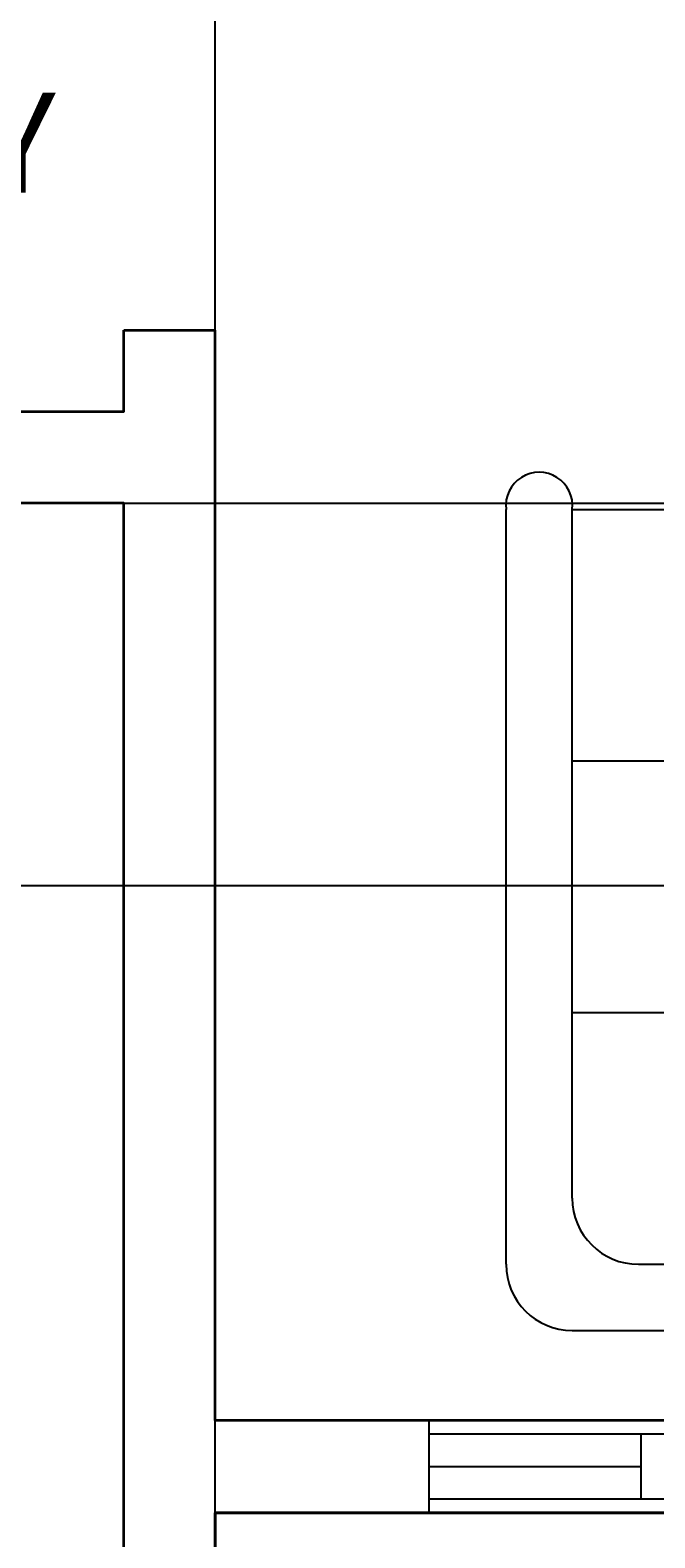
# Model space of a CAD drawing. Units: millimetres. Extents: x 19292 to 100733, y 12374 to 26974.
# Tile 3 of 24: x 26744 to 28279, y 14845 to 18550. Entities that reach past the tile are written whole.
import ezdxf

# ---------------------------------------------------------------- set-up
doc = ezdxf.new("R2010")
doc.units = ezdxf.units.MM
for name, color, linetype, lineweight in [('A-ANNO-DIMS', 2, 'Continuous', 18), ('A-AREA-IDEN', 3, 'Continuous', 25), ('A-FLOR-PATT', 252, 'Continuous', 13), ('A-FURN', 8, 'Continuous', 18), ('A-GLAZ', 3, 'Continuous', 25), ('A-WALL', 7, 'Continuous', 35)]:
    doc.layers.add(name, color=color, linetype=linetype, lineweight=lineweight)
doc.layers.add('FURNITURE', color=40, linetype='Continuous')
doc.layers.add('WINDOWS', color=50, linetype='Continuous')
doc.styles.get("Standard").update_dxf_attribs({"font": 'arial.ttf'})
doc.dimstyles.get("Standard").update_dxf_attribs({"dimtxt": 0.18, "dimasz": 0.18, "dimexe": 0.18, "dimexo": 0.0625, "dimgap": 0.09, "dimtad": 0, "dimtih": 1, "dimtoh": 1, "dimdec": 4, "dimzin": 0, "dimdsep": 46, "dimtxsty": 'Standard', "dimcen": 0.09, "dimadec": 0, "dimazin": 0, "dimtfac": 1, "dimtdec": 4, "dimtofl": 0, "dimtmove": 0, "dimatfit": 3, "dimfxl": 1, "dimtolj": 1, "dimtzin": 0, "dimarcsym": 0})

# ---------------------------------------------------------------- blocks, each defined once
blk = doc.blocks.new('WW')
at = {"layer": 'WINDOWS'}
for p, q in [((-5183.9, -4940.9), (-3983.9, -4940.9)), ((-4663.9, -4940.9), (-4663.9, -5100.9)), ((-4503.9, -4940.9), (-4503.9, -5100.9)), ((-4503.9, -4940.9), (-4503.9, -5100.9)), ((-5183.9, -5020.9), (-4663.9, -5020.9)), ((-4503.9, -5020.9), (-3983.9, -5020.9)), ((-5183.9, -5100.9), (-3983.9, -5100.9))]:
    blk.add_line(p, q, dxfattribs=at)
for points in [[(-5183.9, -5133.4), (-5183.9, -4908.4)], [(-3983.9, -4908.4), (-3983.9, -5133.4)]]:
    blk.add_lwpolyline(points, dxfattribs=at)
blk = doc.blocks.new('2sofa-hf')
at = {"layer": 'FURNITURE'}
for p, q in [((-27, -29.85), (-27, 31.72)), ((-21.6, -24.45), (-21.6, 31.72)), ((-21.6, 31.72), (-13.69, 31.72)), ((0, -6.32), (0, 19.35)), ((-21.62, 11.2), (-0.02, 11.2)), ((-21.57, -9.32), (-2.97, -9.32)), ((0, -23.85), (0, -12.32)), ((-16.2, -29.85), (-3, -29.85)), ((-21.6, -35.25), (-2.43, -35.25))]:
    blk.add_line(p, q, dxfattribs=at)
for centre, radius, start, end in [((-24.3, 32.03), 2.72, 353.479, 186.521), ((-11.92, 19.92), 11.93, 357.2261, 98.5207), ((-3, -6.32), 3, 270, 0), ((-3, -12.32), 3, 0, 90), ((-16.2, -24.45), 5.4, 180, 270), ((-6, -23.85), 6, 270, 0), ((-21.6, -29.85), 5.4, 180, 270), ((-2.71, -32.55), 2.72, 263.9744, 96.0256)]:
    blk.add_arc(centre, radius, start, end, dxfattribs=at)
blk = doc.blocks.new('*D70')
at = {"layer": 'A-ANNO-DIMS', "color": 0, "lineweight": -2, "transparency": 16777216}
for p, q in [((23573.9, 17387.7), (36879.3, 17387.7)), ((36879.2, 17387.6), (36879.2, 16917.9)), ((36879.2, 16447.9), (36879.2, 16917.6)), ((23573.9, 16447.7), (36879.3, 16447.7))]:
    blk.add_line(p, q, dxfattribs=at)
at = {"layer": 'A-ANNO-DIMS', "color": 0, "transparency": 16777216}
for points in [[(36879.1, 17387.6), (36879.2, 17387.6), (36879.2, 17387.7)], [(36879.1, 16447.9), (36879.2, 16447.9), (36879.2, 16447.7)]]:
    blk.add_solid(points, dxfattribs=at)
at = {"layer": 'Defpoints', "color": 0, "transparency": 16777216}
for p in [(23573.8, 17387.7), (36879.2, 17387.7), (23573.8, 16447.7)]:
    blk.add_point(p, dxfattribs=at)
at = {"layer": 'A-ANNO-DIMS', "color": 0, "transparency": 16777216, "insert": (36879.2, 16917.7), "char_height": 0.18, "attachment_point": 5}
blk.add_mtext('\\A1;940', dxfattribs=at)
blk = doc.blocks.new('*D71')
at = {"layer": 'A-ANNO-DIMS', "color": 0, "lineweight": -2, "transparency": 16777216}
for p, q in [((26973.8, 17387.7), (26278.6, 17387.7)), ((26278.8, 17387.6), (26278.8, 15587.9)), ((26278.8, 13787.9), (26278.8, 15587.6)), ((26973.8, 13787.7), (26278.6, 13787.7))]:
    blk.add_line(p, q, dxfattribs=at)
at = {"layer": 'A-ANNO-DIMS', "color": 0, "transparency": 16777216}
for points in [[(26278.8, 17387.6), (26278.8, 17387.6), (26278.8, 17387.7)], [(26278.8, 13787.9), (26278.8, 13787.9), (26278.8, 13787.7)]]:
    blk.add_solid(points, dxfattribs=at)
at = {"layer": 'Defpoints', "color": 0, "transparency": 16777216}
for p in [(26278.8, 17387.7), (26973.8, 17387.7), (26973.8, 13787.7)]:
    blk.add_point(p, dxfattribs=at)
at = {"layer": 'A-ANNO-DIMS', "color": 0, "transparency": 16777216, "insert": (26278.8, 15587.7), "char_height": 0.18, "attachment_point": 5}
blk.add_mtext('\\A1;3600', dxfattribs=at)
blk = doc.blocks.new('*D79')
at = {"layer": 'A-ANNO-DIMS', "color": 0, "lineweight": -2, "transparency": 16777216}
for p, q in [((22694.1, 22860.7), (22694.1, 12808.8)), ((36144.2, 15985.7), (36144.2, 12808.8)), ((22694.3, 12809), (29418.7, 12809)), ((36144, 12809), (29419.6, 12809))]:
    blk.add_line(p, q, dxfattribs=at)
at = {"layer": 'A-ANNO-DIMS', "color": 0, "transparency": 16777216}
for points in [[(22694.3, 12809), (22694.3, 12809), (22694.1, 12809)], [(36144, 12809), (36144, 12809), (36144.2, 12809)]]:
    blk.add_solid(points, dxfattribs=at)
at = {"layer": 'Defpoints', "color": 0, "transparency": 16777216}
for p in [(22694.1, 22860.7), (36144.2, 15985.7), (36144.2, 12809)]:
    blk.add_point(p, dxfattribs=at)
at = {"layer": 'A-ANNO-DIMS', "color": 0, "transparency": 16777216, "insert": (29419.2, 12809), "char_height": 0.18, "attachment_point": 5}
blk.add_mtext('\\A1;13450', dxfattribs=at)
blk = doc.blocks.new('*D82')
at = {"layer": 'A-ANNO-DIMS', "color": 0, "lineweight": -2, "transparency": 16777216}
for p, q in [((27198.8, 13562.8), (27198.8, 23555.9)), ((27199, 23555.7), (29296.4, 23555.7)), ((31394.6, 23555.7), (29297.2, 23555.7)), ((31394.8, 13544.1), (31394.8, 23555.9))]:
    blk.add_line(p, q, dxfattribs=at)
at = {"layer": 'A-ANNO-DIMS', "color": 0, "transparency": 16777216}
for points in [[(27199, 23555.8), (27199, 23555.7), (27198.8, 23555.7)], [(31394.6, 23555.8), (31394.6, 23555.7), (31394.8, 23555.7)]]:
    blk.add_solid(points, dxfattribs=at)
at = {"layer": 'Defpoints', "color": 0, "transparency": 16777216}
for p in [(31394.8, 23555.7), (27198.8, 13562.7), (31394.8, 13544)]:
    blk.add_point(p, dxfattribs=at)
at = {"layer": 'A-ANNO-DIMS', "color": 0, "transparency": 16777216, "insert": (29296.8, 23555.7), "char_height": 0.18, "attachment_point": 5}
blk.add_mtext('\\A1;4196', dxfattribs=at)
blk = doc.blocks.new('*D86')
at = {"layer": 'A-ANNO-DIMS', "color": 0, "lineweight": -2, "transparency": 16777216}
for p, q in [((27198.8, 15132.8), (27198.8, 23555.9)), ((27199, 23555.7), (29198.5, 23555.7)), ((31198.6, 23555.7), (29199.2, 23555.7)), ((31198.8, 15132.8), (31198.8, 23555.9))]:
    blk.add_line(p, q, dxfattribs=at)
at = {"layer": 'A-ANNO-DIMS', "color": 0, "transparency": 16777216}
for points in [[(27199, 23555.8), (27199, 23555.7), (27198.8, 23555.7)], [(31198.6, 23555.8), (31198.6, 23555.7), (31198.8, 23555.7)]]:
    blk.add_solid(points, dxfattribs=at)
at = {"layer": 'Defpoints', "color": 0, "transparency": 16777216}
for p in [(31198.8, 23555.7), (27198.8, 15132.7), (31198.8, 15132.7)]:
    blk.add_point(p, dxfattribs=at)
at = {"layer": 'A-ANNO-DIMS', "color": 0, "transparency": 16777216, "insert": (29198.8, 23555.7), "char_height": 0.18, "attachment_point": 5}
blk.add_mtext('\\A1;4000', dxfattribs=at)

msp = doc.modelspace()

# ---------------------------------------------------------------- hatches: boundary and pattern name
at = {"layer": 'A-FLOR-PATT'}
h = msp.add_hatch(dxfattribs=at)
h.set_pattern_fill('CROSS', color=256, scale=40)
h.paths.add_polyline_path([(31394.799, 14906.403), (31051.542, 14906.403), (29468.571, 14906.403), (27198.815, 14906.403), (27198.815, 13543.993), (31394.799, 13543.993)])
h.paths.add_polyline_path([(27828.096, 14036.581), (30629.164, 14036.581), (30629.164, 14443.478), (27828.096, 14443.478)], flags=24)

# ---------------------------------------------------------------- linework, layer by layer
at = {"layer": 'A-WALL'}
msp.add_line((26973.815, 17812.748), (27198.815, 17812.748), dxfattribs=at)
for points in [[(29548.571, 14906.403), (27198.815, 14906.403), (27198.815, 13562.748), (23348.815, 13562.748), (23348.815, 19010.725), (22694.132, 19010.725), (22694.132, 22860.725), (28369.132, 22860.725), (28369.132, 21460.725), (31169.132, 21460.725), (31169.132, 22460.725), (34419.132, 22460.725), (34419.132, 22208.026)], [(26576.145, 17612.748), (26973.815, 17612.748), (26973.815, 17812.748)], [(29468.571, 15132.748), (27198.815, 15132.748), (27198.815, 17812.748)], [(25756.145, 17387.748), (23573.815, 17387.748), (23573.815, 13787.748), (26973.815, 13787.748), (26973.815, 17387.748), (26656.145, 17387.748)], [(31051.542, 14906.403), (31394.799, 14906.403), (31394.799, 13543.993), (27198.815, 13543.993), (27198.815, 14906.403), (29548.571, 14906.403)]]:
    msp.add_lwpolyline(points, dxfattribs=at)

# ---------------------------------------------------------------- block references
at = {"layer": 'A-FURN', "xscale": 30.13269765108242, "yscale": 30.13269765108242, "zscale": 30.13269765108242}
msp.add_blockref('2sofa-hf', (28726.739, 16416.302), dxfattribs=at)
at = {"layer": 'A-GLAZ'}
msp.add_blockref('WW', (32907.943, 20041.124), dxfattribs=at)

# ---------------------------------------------------------------- texts
at = {"layer": 'A-AREA-IDEN'}
msp.add_text('LOBBY', height=245.412, dxfattribs=at).set_placement((25758.801, 18150.521))

# ---------------------------------------------------------------- dimensions: what is measured, and where the dimension line sits
at = {"layer": 'A-ANNO-DIMS'}
for base, p1, p2, picture, middle in [((31394.799, 23555.725), (27198.815, 13562.748), (31394.799, 13543.993), '*D82', (29296.807, 23555.725)), ((31198.815, 23555.725), (27198.815, 15132.748), (31198.815, 15132.748), '*D86', (29198.815, 23555.725)), ((36144.169, 12808.993), (22694.132, 22860.725), (36144.169, 15985.725), '*D79', (29419.151, 12808.993))]:
    dim = msp.add_linear_dim(base=base, p1=p1, p2=p2, dimstyle='Standard', override={"dimdec": 0, "dimlfac": 1, "dimrnd": 0, "dimzin": 0, "dimdsep": 46, "dimlunit": 2}, dxfattribs=at)
    dim.commit()
    dim.dimension.update_dxf_attribs({"geometry": picture, "text_midpoint": middle})
for base, p1, p2, picture, middle in [((36879.169, 17387.748), (23573.815, 16447.748), (23573.815, 17387.748), '*D70', (36879.169, 16917.748)), ((26278.815, 17387.748), (26973.815, 13787.748), (26973.815, 17387.748), '*D71', (26278.815, 15587.748))]:
    dim = msp.add_linear_dim(base=base, p1=p1, p2=p2, angle=90, dimstyle='Standard', override={"dimdec": 0, "dimlfac": 1, "dimrnd": 0, "dimzin": 0, "dimdsep": 46, "dimlunit": 2}, dxfattribs=at)
    dim.commit()
    dim.dimension.update_dxf_attribs({"geometry": picture, "text_midpoint": middle})

doc.saveas('drawing.dxf')
